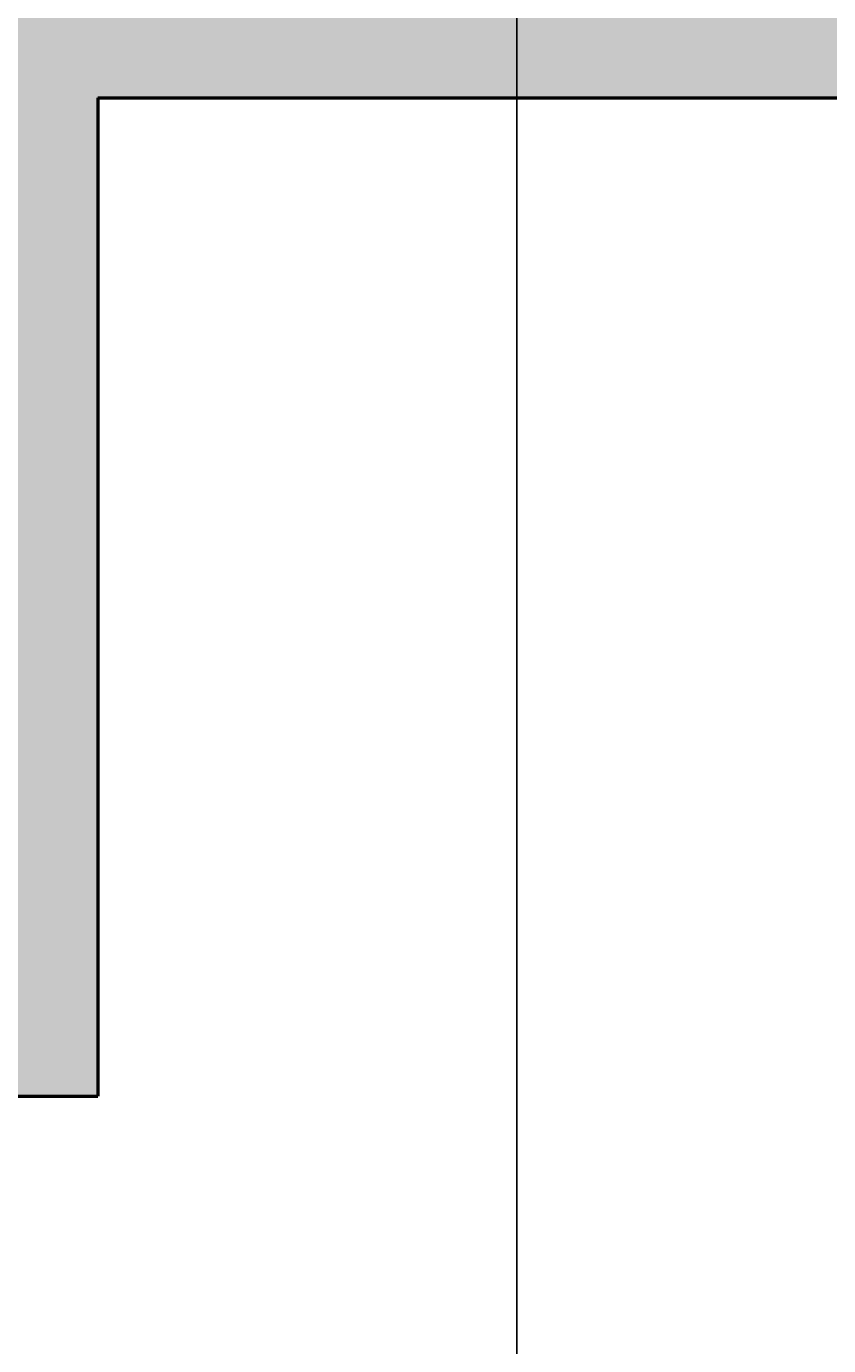
# Model space of a CAD drawing. Units: inches. Extents: x 2231 to 2461, y 2045 to 2455.
# Tile 63 of 95: x 2371 to 2393, y 2296 to 2333. Entities that reach past the tile are written whole.
import ezdxf

# ---------------------------------------------------------------- set-up
doc = ezdxf.new("R2010")
doc.units = ezdxf.units.IN
doc.layers.add('A-ANNO-DIMS', color=2, linetype='Continuous', lineweight=18)
doc.layers.add('A-WALL', color=7, linetype='Continuous', lineweight=50)
doc.layers.add('A-WALL-PATT', color=18, linetype='Continuous', lineweight=13, true_color=0x000000)
doc.styles.get("Standard").update_dxf_attribs({"font": 'arial.ttf'})
doc.dimstyles.get("Standard").update_dxf_attribs({"dimtxt": 0.18, "dimasz": 0.18, "dimexe": 0.18, "dimexo": 0.0625, "dimgap": 0.09, "dimtad": 0, "dimtih": 1, "dimtoh": 1, "dimdec": 4, "dimzin": 0, "dimdsep": 46, "dimtxsty": 'Standard', "dimcen": 0.09, "dimadec": 0, "dimazin": 0, "dimtfac": 1, "dimtdec": 4, "dimtofl": 0, "dimtmove": 0, "dimatfit": 3, "dimfxl": 1, "dimtolj": 1, "dimtzin": 0, "dimarcsym": 0})

# ---------------------------------------------------------------- blocks, each defined once
blk = doc.blocks.new('*D66')
at = {"layer": 'A-ANNO-DIMS', "color": 0, "lineweight": -2, "transparency": 16777216}
for p, q in [((2348.189, 2096.895), (2348.189, 2454.645)), ((2408.794, 2096.895), (2408.794, 2454.645)), ((2348.369, 2454.465), (2378.167, 2454.465)), ((2408.614, 2454.465), (2378.815, 2454.465))]:
    blk.add_line(p, q, dxfattribs=at)
at = {"layer": 'A-ANNO-DIMS', "color": 0, "transparency": 16777216}
for points in [[(2348.369, 2454.495), (2348.369, 2454.435), (2348.189, 2454.465)], [(2408.614, 2454.495), (2408.614, 2454.435), (2408.794, 2454.465)]]:
    blk.add_solid(points, dxfattribs=at)
at = {"layer": 'Defpoints', "color": 0, "transparency": 16777216}
for p in [(2408.794, 2454.465), (2348.189, 2096.833), (2408.794, 2096.833)]:
    blk.add_point(p, dxfattribs=at)
at = {"layer": 'A-ANNO-DIMS', "color": 0, "transparency": 16777216, "insert": (2378.491, 2454.465), "char_height": 0.18, "attachment_point": 5}
blk.add_mtext('\\A1;60.6', dxfattribs=at)
blk = doc.blocks.new('*D72')
at = {"layer": 'A-ANNO-DIMS', "color": 0, "lineweight": -2, "transparency": 16777216}
for p, q in [((2384.543, 2145.12), (2384.543, 2454.645)), ((2408.794, 2150.677), (2408.794, 2454.645)), ((2384.723, 2454.465), (2396.272, 2454.465)), ((2408.614, 2454.465), (2397.064, 2454.465))]:
    blk.add_line(p, q, dxfattribs=at)
at = {"layer": 'A-ANNO-DIMS', "color": 0, "transparency": 16777216}
for points in [[(2384.723, 2454.495), (2384.723, 2454.435), (2384.543, 2454.465)], [(2408.614, 2454.495), (2408.614, 2454.435), (2408.794, 2454.465)]]:
    blk.add_solid(points, dxfattribs=at)
at = {"layer": 'Defpoints', "color": 0, "transparency": 16777216}
for p in [(2408.794, 2454.465), (2408.794, 2150.615), (2384.543, 2145.058)]:
    blk.add_point(p, dxfattribs=at)
at = {"layer": 'A-ANNO-DIMS', "color": 0, "transparency": 16777216, "insert": (2396.668, 2454.465), "char_height": 0.18, "attachment_point": 5}
blk.add_mtext('\\A1;24.25', dxfattribs=at)

msp = doc.modelspace()

# ---------------------------------------------------------------- hatches: boundary and pattern name
at = {"layer": 'A-WALL-PATT'}
h = msp.add_hatch(color=256, dxfattribs=at)
h.dxf.hatch_style = 1
h.paths.add_polyline_path([(2441.7935, 2269.1535), (2432.7935, 2269.1535), (2432.7935, 2186.8328), (2396.7935, 2186.8328), (2396.7935, 2286.8328), (2394.7935, 2286.8328), (2394.7935, 2186.8328), (2334.7935, 2186.8328), (2334.7935, 2182.8328), (2432.7935, 2182.8328), (2432.7935, 2072.8328), (2416.6639, 2072.8328), (2416.6639, 2063.8328), (2441.7935, 2063.8328)])
h.paths.add_polyline_path([(2368.6639, 2072.8328), (2367.04, 2072.8328), (2330.7942, 2072.8328), (2330.7397, 2063.8328), (2368.6639, 2063.8328)])
h.paths.add_polyline_path([(2300.7392, 2068.3328), (2300.7392, 2072.8328), (2298.7935, 2072.8328), (2294.7935, 2072.8328), (2258.7935, 2072.8328), (2258.7935, 2120.8328), (2294.7935, 2120.8328), (2298.7935, 2120.8328), (2298.7935, 2128.8328), (2294.7935, 2128.8328), (2294.7935, 2124.8328), (2258.7935, 2124.8328), (2258.7935, 2182.8328), (2294.7935, 2182.8328), (2294.7935, 2174.8328), (2298.7935, 2174.8328), (2298.7935, 2182.8328), (2304.7935, 2182.8328), (2304.7935, 2186.8328), (2258.7935, 2186.8328), (2258.7935, 2221.999), (2249.7935, 2221.999), (2249.7935, 2063.8328), (2300.7392, 2063.8328)])
h.paths.add_polyline_path([(2391.9338, 2435.8328), (2333.82, 2435.8328), (2333.82, 2426.8328), (2368.7935, 2426.8328), (2368.7935, 2374.9508), (2368.7935, 2370.8328), (2372.3935, 2370.8328), (2372.7935, 2370.8328), (2372.7935, 2426.8328), (2391.9338, 2426.8328)])
h.paths.add_polyline_path([(2441.7935, 2435.8328), (2415.9338, 2435.8328), (2415.9338, 2426.8328), (2432.7935, 2426.8328), (2432.7935, 2334.8328), (2372.7935, 2334.8328), (2372.7935, 2346.8328), (2368.7935, 2346.8328), (2368.7935, 2306.8328), (2360.7935, 2306.8328), (2360.7935, 2302.8328), (2368.7935, 2302.8328), (2372.7935, 2302.8328), (2372.7935, 2330.8328), (2432.7935, 2330.8328), (2432.7935, 2317.1535), (2441.7935, 2317.1535)])
h.paths.add_polyline_path([(2285.82, 2435.8328), (2249.7935, 2435.8328), (2249.7935, 2269.999), (2258.7935, 2269.999), (2258.7935, 2302.8328), (2318.8168, 2302.8328), (2330.7935, 2302.8328), (2330.7935, 2306.8328), (2258.7935, 2306.8328), (2258.7935, 2426.8328), (2285.82, 2426.8328)])

# ---------------------------------------------------------------- linework, layer by layer
at = {"layer": 'A-WALL'}
for p, q in [((2372.7935, 2330.8328), (2432.7935, 2330.8328)), ((2372.7935, 2330.8328), (2372.7935, 2302.8328)), ((2368.7935, 2302.8328), (2372.7935, 2302.8328))]:
    msp.add_line(p, q, dxfattribs=at)

# ---------------------------------------------------------------- dimensions: what is measured, and where the dimension line sits
at = {"layer": 'A-ANNO-DIMS'}
for p1, p2, override, picture, middle in [((2348.1888, 2096.8328), (2408.7935, 2096.8328), {"dimdec": 1, "dimlfac": 1, "dimrnd": 0, "dimzin": 0, "dimdsep": 46, "dimlunit": 2}, '*D66', (2378.4912, 2454.4653)), ((2384.5428, 2145.0576), (2408.7935, 2150.6145), {"dimdec": 2, "dimlfac": 1, "dimrnd": 0, "dimzin": 0, "dimdsep": 46, "dimlunit": 2}, '*D72', (2396.6682, 2454.4653))]:
    dim = msp.add_linear_dim(base=(2408.7935, 2454.4653), p1=p1, p2=p2, dimstyle='Standard', override=override, dxfattribs=at)
    dim.commit()
    dim.dimension.update_dxf_attribs({"geometry": picture, "text_midpoint": middle})

doc.saveas('drawing.dxf')
